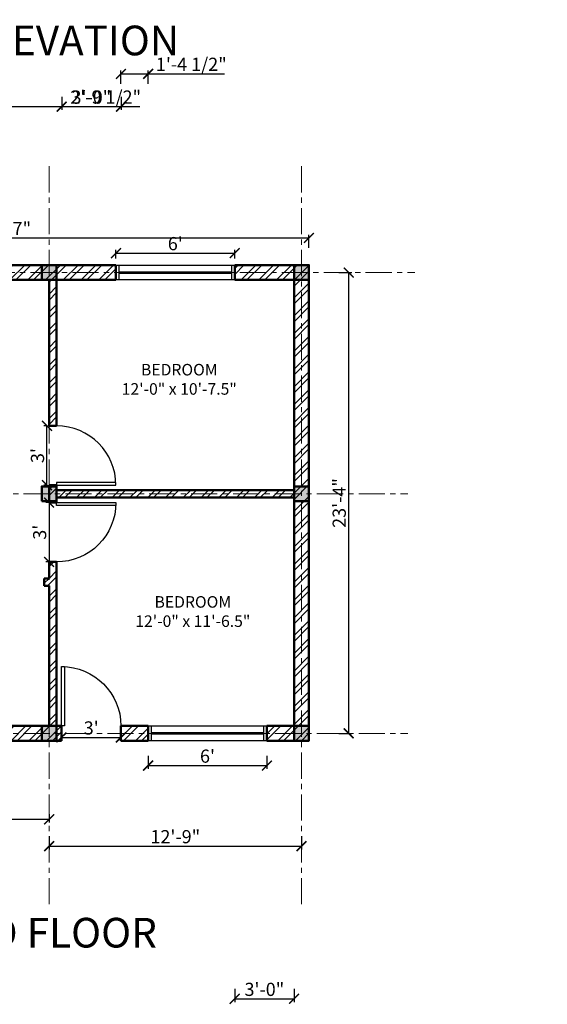
# Model space of a CAD drawing. Units: inches. Extents: x 378 to 1617, y 130 to 1256.
# Tile 2 of 5: x 708 to 1028, y 134 to 731. Entities that reach past the tile are written whole.
import ezdxf

# ---------------------------------------------------------------- set-up
doc = ezdxf.new("R2010")
doc.units = ezdxf.units.IN
doc.linetypes.add('CENTER', pattern=[50.8, 31.75, -6.35, 6.35, -6.35])
for name, color, linetype, lineweight in [('A-ANNO-TEXT', 7, 'Continuous', 25), ('A-AREA-IDEN', 3, 'Continuous', 18), ('Column Hatch', 1, 'Continuous', 13), ('Columns', 241, 'Continuous', 50), ('Dimensions', 153, 'Continuous', 18), ('Doors', 2, 'Continuous', 25), ('Grid lines', 7, 'CENTER', 18), ('Wall Hatch', 11, 'Continuous', 13), ('Walls', 220, 'Continuous', 50), ('Windows', 140, 'Continuous', 25)]:
    doc.layers.add(name, color=color, linetype=linetype, lineweight=lineweight)
doc.styles.get("Standard").update_dxf_attribs({"font": 'arial.ttf'})
doc.dimstyles.new('ISO-25', dxfattribs={"dimtxt": 8, "dimasz": 6, "dimexe": 2, "dimexo": 4, "dimtad": 1, "dimdec": 0, "dimlunit": 3, "dimtxsty": 'Standard', "dimblk": 'ARCHTICK', "dimcen": 2.5, "dimadec": 0, "dimazin": 0, "dimtfac": 1, "dimtdec": 0, "dimtmove": 0, "dimatfit": 3, "dimfxl": 6, "dimfxlon": 1, "dimarcsym": 0})

# ---------------------------------------------------------------- blocks, each defined once
blk = doc.blocks.new('*U5')
for p, q in [((0, 0), (0, -4)), ((-36, 0), (-36, -4))]:
    blk.add_line(p, q)
blk.add_lwpolyline([(0, 0), (0, 36), (-1.75, 36), (-1.75, 0)], close=True)
blk.add_arc((0, 0), 36, 90, 180)
blk = doc.blocks.new('*U6')
for p, q in [((0, 0), (0, -4)), ((-36, 0), (-36, -4))]:
    blk.add_line(p, q)
blk.add_lwpolyline([(0, 0), (0, 36), (-1.75, 36), (-1.75, 0)], close=True)
blk.add_arc((0, 0), 36, 90, 180)
blk = doc.blocks.new('_ArchTick')
at = {"color": 0, "linetype": 'ByBlock', "const_width": 0.15}
blk.add_lwpolyline([(-0.5, -0.5), (0.5, 0.5)], dxfattribs=at)
blk = doc.blocks.new('*D9')
at = {"layer": 'Defpoints', "color": 0, "transparency": 16777216}
for p in [(614.03, 252.95), (726.03, 252.95), (726.03, 245.84)]:
    blk.add_point(p, dxfattribs=at)
at = {"layer": 'Dimensions', "color": 0, "lineweight": -2, "transparency": 16777216}
for p, q in [((614.03, 248.95), (614.03, 243.84)), ((614.03, 245.84), (726.03, 245.84)), ((726.03, 248.95), (726.03, 243.84))]:
    blk.add_line(p, q, dxfattribs=at)
at = {"layer": 'Dimensions', "color": 0, "lineweight": -2, "transparency": 16777216, "xscale": 6, "yscale": 6, "zscale": 6, "rotation": 180}
blk.add_blockref('_ArchTick', (614.03, 245.84), dxfattribs=at)
at = {"layer": 'Dimensions', "color": 0, "lineweight": -2, "transparency": 16777216, "xscale": 6, "yscale": 6, "zscale": 6}
blk.add_blockref('_ArchTick', (726.03, 245.84), dxfattribs=at)
at = {"layer": 'Dimensions', "color": 0, "transparency": 16777216, "insert": (670.03, 250.55), "char_height": 8, "attachment_point": 5}
blk.add_mtext('9\'-4"', dxfattribs=at)
blk = doc.blocks.new('*D10')
at = {"layer": 'Defpoints', "color": 0, "transparency": 16777216}
for p in [(726.03, 293.45), (879.03, 293.45), (879.03, 229.55)]:
    blk.add_point(p, dxfattribs=at)
at = {"layer": 'Dimensions', "color": 0, "lineweight": -2, "transparency": 16777216}
for p, q in [((726.03, 235.55), (726.03, 227.55)), ((879.03, 235.55), (879.03, 227.55)), ((726.03, 229.55), (879.03, 229.55))]:
    blk.add_line(p, q, dxfattribs=at)
at = {"layer": 'Dimensions', "color": 0, "lineweight": -2, "transparency": 16777216, "xscale": 6, "yscale": 6, "zscale": 6, "rotation": 180}
blk.add_blockref('_ArchTick', (726.03, 229.55), dxfattribs=at)
at = {"layer": 'Dimensions', "color": 0, "lineweight": -2, "transparency": 16777216, "xscale": 6, "yscale": 6, "zscale": 6}
blk.add_blockref('_ArchTick', (879.03, 229.55), dxfattribs=at)
at = {"layer": 'Dimensions', "color": 0, "transparency": 16777216, "insert": (802.53, 234.26), "char_height": 8, "attachment_point": 5}
blk.add_mtext('12\'-9"', dxfattribs=at)
blk = doc.blocks.new('*D13')
at = {"layer": 'Defpoints', "color": 0, "transparency": 16777216}
for p in [(883.53, 577.45), (907.65, 577.45), (883.53, 297.95)]:
    blk.add_point(p, dxfattribs=at)
at = {"layer": 'Dimensions', "color": 0, "lineweight": -2, "transparency": 16777216}
for p, q in [((901.65, 577.45), (909.65, 577.45)), ((907.65, 297.95), (907.65, 577.45)), ((901.65, 297.95), (909.65, 297.95))]:
    blk.add_line(p, q, dxfattribs=at)
at = {"layer": 'Dimensions', "color": 0, "lineweight": -2, "transparency": 16777216, "xscale": 6, "yscale": 6, "zscale": 6}
for p, rotation in [((907.65, 577.45), 90), ((907.65, 297.95), 270)]:
    blk.add_blockref('_ArchTick', p, dxfattribs=dict(at, rotation=rotation))
at = {"layer": 'Dimensions', "color": 0, "transparency": 16777216, "insert": (902.94, 437.7), "char_height": 8, "attachment_point": 5, "rotation": 90}
blk.add_mtext('23\'-4"', dxfattribs=at)
blk = doc.blocks.new('*D14')
at = {"layer": 'Defpoints', "color": 0, "transparency": 16777216}
for p in [(883.53, 598.41), (516.53, 581.95), (883.53, 581.95)]:
    blk.add_point(p, dxfattribs=at)
at = {"layer": 'Dimensions', "color": 0, "lineweight": -2, "transparency": 16777216}
for p, q in [((516.53, 592.41), (516.53, 600.41)), ((516.53, 598.41), (883.53, 598.41)), ((883.53, 592.41), (883.53, 600.41))]:
    blk.add_line(p, q, dxfattribs=at)
at = {"layer": 'Dimensions', "color": 0, "lineweight": -2, "transparency": 16777216, "xscale": 6, "yscale": 6, "zscale": 6, "rotation": 180}
blk.add_blockref('_ArchTick', (516.53, 598.41), dxfattribs=at)
at = {"layer": 'Dimensions', "color": 0, "lineweight": -2, "transparency": 16777216, "xscale": 6, "yscale": 6, "zscale": 6}
blk.add_blockref('_ArchTick', (883.53, 598.41), dxfattribs=at)
at = {"layer": 'Dimensions', "color": 0, "transparency": 16777216, "insert": (700.03, 603.12), "char_height": 8, "attachment_point": 5}
blk.add_mtext('30\'-7"', dxfattribs=at)
blk = doc.blocks.new('*D26')
at = {"layer": 'Defpoints', "color": 0, "transparency": 16777216}
for p in [(838.53, 589.23), (766.53, 581.95), (838.53, 581.95)]:
    blk.add_point(p, dxfattribs=at)
at = {"layer": 'Dimensions', "color": 0, "lineweight": -2, "transparency": 16777216}
for p, q in [((766.53, 585.95), (766.53, 591.23)), ((838.53, 585.95), (838.53, 591.23)), ((766.53, 589.23), (838.53, 589.23))]:
    blk.add_line(p, q, dxfattribs=at)
at = {"layer": 'Dimensions', "color": 0, "lineweight": -2, "transparency": 16777216, "xscale": 6, "yscale": 6, "zscale": 6, "rotation": 180}
blk.add_blockref('_ArchTick', (766.53, 589.23), dxfattribs=at)
at = {"layer": 'Dimensions', "color": 0, "lineweight": -2, "transparency": 16777216, "xscale": 6, "yscale": 6, "zscale": 6}
blk.add_blockref('_ArchTick', (838.53, 589.23), dxfattribs=at)
at = {"layer": 'Dimensions', "color": 0, "transparency": 16777216, "insert": (802.53, 593.94), "char_height": 8, "attachment_point": 5}
blk.add_mtext("6'", dxfattribs=at)
blk = doc.blocks.new('*D27')
at = {"layer": 'Defpoints', "color": 0, "transparency": 16777216}
for p in [(786.03, 293.45), (858.03, 293.45), (858.03, 278.41)]:
    blk.add_point(p, dxfattribs=at)
at = {"layer": 'Dimensions', "color": 0, "lineweight": -2, "transparency": 16777216}
for p, q in [((786.03, 284.41), (786.03, 276.41)), ((858.03, 284.41), (858.03, 276.41)), ((786.03, 278.41), (858.03, 278.41))]:
    blk.add_line(p, q, dxfattribs=at)
at = {"layer": 'Dimensions', "color": 0, "lineweight": -2, "transparency": 16777216, "xscale": 6, "yscale": 6, "zscale": 6, "rotation": 180}
blk.add_blockref('_ArchTick', (786.03, 278.41), dxfattribs=at)
at = {"layer": 'Dimensions', "color": 0, "lineweight": -2, "transparency": 16777216, "xscale": 6, "yscale": 6, "zscale": 6}
blk.add_blockref('_ArchTick', (858.03, 278.41), dxfattribs=at)
at = {"layer": 'Dimensions', "color": 0, "transparency": 16777216, "insert": (822.03, 283.12), "char_height": 8, "attachment_point": 5}
blk.add_mtext("6'", dxfattribs=at)
blk = doc.blocks.new('*D29')
at = {"layer": 'Defpoints', "color": 0, "transparency": 16777216}
for p in [(733.53, 297.95), (769.53, 297.95), (769.53, 295.49)]:
    blk.add_point(p, dxfattribs=at)
at = {"layer": 'Dimensions', "color": 0, "lineweight": -2, "transparency": 16777216}
for p, q in [((733.53, 295.49), (733.53, 293.49)), ((733.53, 295.49), (769.53, 295.49)), ((769.53, 295.49), (769.53, 293.49))]:
    blk.add_line(p, q, dxfattribs=at)
at = {"layer": 'Dimensions', "color": 0, "lineweight": -2, "transparency": 16777216, "xscale": 6, "yscale": 6, "zscale": 6, "rotation": 180}
blk.add_blockref('_ArchTick', (733.53, 295.49), dxfattribs=at)
at = {"layer": 'Dimensions', "color": 0, "lineweight": -2, "transparency": 16777216, "xscale": 6, "yscale": 6, "zscale": 6}
blk.add_blockref('_ArchTick', (769.53, 295.49), dxfattribs=at)
at = {"layer": 'Dimensions', "color": 0, "transparency": 16777216, "insert": (751.53, 300.21), "char_height": 8, "attachment_point": 5}
blk.add_mtext("3'", dxfattribs=at)
blk = doc.blocks.new('*D30')
at = {"layer": 'Defpoints', "color": 0, "transparency": 16777216}
for p in [(728.53, 437.95), (726.03, 401.95), (728.53, 401.95)]:
    blk.add_point(p, dxfattribs=at)
at = {"layer": 'Dimensions', "color": 0, "lineweight": -2, "transparency": 16777216}
for p, q in [((726.03, 437.95), (724.03, 437.95)), ((726.03, 437.95), (726.03, 401.95)), ((726.03, 401.95), (724.03, 401.95))]:
    blk.add_line(p, q, dxfattribs=at)
at = {"layer": 'Dimensions', "color": 0, "lineweight": -2, "transparency": 16777216, "xscale": 6, "yscale": 6, "zscale": 6}
for p, rotation in [((726.03, 437.95), 90), ((726.03, 401.95), 270)]:
    blk.add_blockref('_ArchTick', p, dxfattribs=dict(at, rotation=rotation))
at = {"layer": 'Dimensions', "color": 0, "transparency": 16777216, "insert": (721.32, 419.95), "char_height": 8, "attachment_point": 5, "rotation": 90}
blk.add_mtext("3'", dxfattribs=at)
blk = doc.blocks.new('*D34')
at = {"layer": 'Defpoints', "color": 0, "transparency": 16777216}
for p in [(724.72, 484.45), (728.28, 484.45), (728.28, 448.45)]:
    blk.add_point(p, dxfattribs=at)
at = {"layer": 'Dimensions', "color": 0, "lineweight": -2, "transparency": 16777216}
for p, q in [((724.72, 484.45), (722.72, 484.45)), ((724.72, 448.45), (724.72, 484.45)), ((724.72, 448.45), (722.72, 448.45))]:
    blk.add_line(p, q, dxfattribs=at)
at = {"layer": 'Dimensions', "color": 0, "lineweight": -2, "transparency": 16777216, "xscale": 6, "yscale": 6, "zscale": 6}
for p, rotation in [((724.72, 484.45), 90), ((724.72, 448.45), 270)]:
    blk.add_blockref('_ArchTick', p, dxfattribs=dict(at, rotation=rotation))
at = {"layer": 'Dimensions', "color": 0, "transparency": 16777216, "insert": (720.01, 466.45), "char_height": 8, "attachment_point": 5, "rotation": 90}
blk.add_mtext("3'", dxfattribs=at)
blk = doc.blocks.new('*D58')
at = {"layer": 'Defpoints', "color": 0, "transparency": 16777216}
for p in [(838.53, 572.95), (874.53, 572.95), (874.53, 136.95)]:
    blk.add_point(p, dxfattribs=at)
at = {"layer": 'Dimensions', "color": 0, "lineweight": -2, "transparency": 16777216}
for p, q in [((838.53, 142.95), (838.53, 134.95)), ((874.53, 142.95), (874.53, 134.95)), ((838.53, 136.95), (874.53, 136.95))]:
    blk.add_line(p, q, dxfattribs=at)
at = {"layer": 'Dimensions', "color": 0, "lineweight": -2, "transparency": 16777216, "xscale": 6, "yscale": 6, "zscale": 6, "rotation": 180}
blk.add_blockref('_ArchTick', (838.53, 136.95), dxfattribs=at)
at = {"layer": 'Dimensions', "color": 0, "lineweight": -2, "transparency": 16777216, "xscale": 6, "yscale": 6, "zscale": 6}
blk.add_blockref('_ArchTick', (874.53, 136.95), dxfattribs=at)
at = {"layer": 'Dimensions', "color": 0, "transparency": 16777216, "insert": (856.53, 141.66), "char_height": 8, "attachment_point": 5}
blk.add_mtext('3\'-0"', dxfattribs=at)
blk = doc.blocks.new('*D60')
at = {"layer": 'Defpoints', "color": 0, "transparency": 16777216}
for p in [(786.03, 697.95), (769.53, 302.45), (786.03, 302.45)]:
    blk.add_point(p, dxfattribs=at)
at = {"layer": 'Dimensions', "color": 0, "lineweight": -2, "transparency": 16777216}
for p, q in [((769.53, 691.95), (769.53, 699.95)), ((786.03, 691.95), (786.03, 699.95)), ((769.53, 697.95), (786.03, 697.95)), ((786.03, 697.95), (832.43, 697.95))]:
    blk.add_line(p, q, dxfattribs=at)
at = {"layer": 'Dimensions', "color": 0, "lineweight": -2, "transparency": 16777216, "xscale": 6, "yscale": 6, "zscale": 6, "rotation": 180}
blk.add_blockref('_ArchTick', (769.53, 697.95), dxfattribs=at)
at = {"layer": 'Dimensions', "color": 0, "lineweight": -2, "transparency": 16777216, "xscale": 6, "yscale": 6, "zscale": 6}
blk.add_blockref('_ArchTick', (786.03, 697.95), dxfattribs=at)
at = {"layer": 'Dimensions', "color": 0, "transparency": 16777216, "insert": (812.23, 702.71), "char_height": 8, "attachment_point": 5}
blk.add_mtext('1\'-4 1/2"', dxfattribs=at)
blk = doc.blocks.new('*D77')
at = {"layer": 'Defpoints', "color": 0, "transparency": 16777216}
for p in [(733.65, 812.09), (769.65, 812.09), (769.65, 678.08)]:
    blk.add_point(p, dxfattribs=at)
at = {"layer": 'Dimensions', "color": 0, "lineweight": -2, "transparency": 16777216}
for p, q in [((733.65, 684.08), (733.65, 676.08)), ((769.65, 684.08), (769.65, 676.08)), ((733.65, 678.08), (769.65, 678.08))]:
    blk.add_line(p, q, dxfattribs=at)
at = {"layer": 'Dimensions', "color": 0, "lineweight": -2, "transparency": 16777216, "xscale": 6, "yscale": 6, "zscale": 6, "rotation": 180}
blk.add_blockref('_ArchTick', (733.65, 678.08), dxfattribs=at)
at = {"layer": 'Dimensions', "color": 0, "lineweight": -2, "transparency": 16777216, "xscale": 6, "yscale": 6, "zscale": 6}
blk.add_blockref('_ArchTick', (769.65, 678.08), dxfattribs=at)
at = {"layer": 'Dimensions', "color": 0, "transparency": 16777216, "insert": (751.65, 682.79), "char_height": 8, "attachment_point": 5}
blk.add_mtext('3\'-0"', dxfattribs=at)
blk = doc.blocks.new('*D82')
at = {"layer": 'Defpoints', "color": 0, "transparency": 16777216}
for p in [(700.03, 851.08), (733.65, 812.09), (733.65, 678.08)]:
    blk.add_point(p, dxfattribs=at)
at = {"layer": 'Dimensions', "color": 0, "lineweight": -2, "transparency": 16777216}
for p, q in [((700.03, 684.08), (700.03, 676.08)), ((733.65, 684.08), (733.65, 676.08)), ((700.03, 678.08), (733.65, 678.08)), ((733.65, 678.08), (780.95, 678.08))]:
    blk.add_line(p, q, dxfattribs=at)
at = {"layer": 'Dimensions', "color": 0, "lineweight": -2, "transparency": 16777216, "xscale": 6, "yscale": 6, "zscale": 6, "rotation": 180}
blk.add_blockref('_ArchTick', (700.03, 678.08), dxfattribs=at)
at = {"layer": 'Dimensions', "color": 0, "lineweight": -2, "transparency": 16777216, "xscale": 6, "yscale": 6, "zscale": 6}
blk.add_blockref('_ArchTick', (733.65, 678.08), dxfattribs=at)
at = {"layer": 'Dimensions', "color": 0, "transparency": 16777216, "insert": (760.3, 682.84), "char_height": 8, "attachment_point": 5}
blk.add_mtext('2\'-9 1/2"', dxfattribs=at)

msp = doc.modelspace()

# ---------------------------------------------------------------- hatches: boundary and pattern name
at = {"layer": 'Column Hatch'}
h = msp.add_hatch(color=256, dxfattribs=at)
h.dxf.hatch_style = 1
h.paths.add_polyline_path([(525.53, 581.95), (516.53, 581.95), (516.53, 572.95), (525.53, 572.95)])
h.paths.add_polyline_path([(618.53, 581.95), (609.53, 581.95), (609.53, 572.95), (618.53, 572.95)])
h.paths.add_polyline_path([(730.53, 581.95), (721.53, 581.95), (721.53, 572.95), (730.53, 572.95)])
h.paths.add_polyline_path([(883.53, 581.95), (874.53, 581.95), (874.53, 572.95), (883.53, 572.95)])
h.paths.add_polyline_path([(883.53, 447.7), (874.53, 447.7), (874.53, 438.7), (883.53, 438.7)])
h.paths.add_polyline_path([(730.53, 447.7), (721.53, 447.7), (721.53, 438.7), (730.53, 438.7)])
h.paths.add_polyline_path([(618.53, 447.7), (609.53, 447.7), (609.53, 438.7), (618.53, 438.7)])
h.paths.add_polyline_path([(525.53, 447.7), (516.53, 447.7), (516.53, 438.7), (525.53, 438.7)])
h.paths.add_polyline_path([(525.53, 302.45), (516.53, 302.45), (516.53, 293.45), (525.53, 293.45)])
h.paths.add_polyline_path([(618.53, 302.45), (609.53, 302.45), (609.53, 293.45), (618.53, 293.45)])
h.paths.add_polyline_path([(730.53, 302.45), (721.53, 302.45), (721.53, 293.45), (730.53, 293.45)])
h.paths.add_polyline_path([(883.53, 302.45), (874.53, 302.45), (874.53, 293.45), (883.53, 293.45)])
h.paths.add_polyline_path([(1125.53, 302.45), (1116.53, 302.45), (1116.53, 293.45), (1125.53, 293.45)])
h.paths.add_polyline_path([(1218.53, 302.45), (1209.53, 302.45), (1209.53, 293.45), (1218.53, 293.45)])
h.paths.add_polyline_path([(1330.53, 302.45), (1321.53, 302.45), (1321.53, 293.45), (1330.53, 293.45)])
h.paths.add_polyline_path([(1483.53, 302.45), (1474.53, 302.45), (1474.53, 293.45), (1483.53, 293.45)])
h.paths.add_polyline_path([(1483.53, 447.7), (1474.53, 447.7), (1474.53, 438.7), (1483.53, 438.7)])
h.paths.add_polyline_path([(1330.53, 447.7), (1321.53, 447.7), (1321.53, 438.7), (1330.53, 438.7)])
h.paths.add_polyline_path([(1218.53, 447.7), (1209.53, 447.7), (1209.53, 438.7), (1218.53, 438.7)])
h.paths.add_polyline_path([(1125.53, 447.7), (1116.53, 447.7), (1116.53, 438.7), (1125.53, 438.7)])
h.paths.add_polyline_path([(1125.53, 581.95), (1116.53, 581.95), (1116.53, 572.95), (1125.53, 572.95)])
h.paths.add_polyline_path([(1218.53, 581.95), (1209.53, 581.95), (1209.53, 572.95), (1218.53, 572.95)])
h.paths.add_polyline_path([(1330.53, 581.95), (1321.53, 581.95), (1321.53, 572.95), (1330.53, 572.95)])
h.paths.add_polyline_path([(1483.53, 581.95), (1474.53, 581.95), (1474.53, 572.95), (1483.53, 572.95)])
at = {"layer": 'Wall Hatch'}
h = msp.add_hatch(dxfattribs=at)
h.set_pattern_fill('ANSI32', color=256, scale=0.8)
h.paths.add_polyline_path([(525.53, 493.45), (609.53, 493.45), (609.53, 490.45), (614.03, 490.45), (614.03, 500.95), (609.53, 500.95), (609.53, 497.95), (525.53, 497.95), (525.53, 572.95), (527.53, 572.95), (527.53, 581.95), (516.53, 581.95), (516.53, 252.95), (614.03, 252.95), (614.03, 293.45), (609.53, 293.45), (609.53, 257.45), (525.53, 257.45), (525.53, 297.95), (609.53, 297.95), (609.53, 302.45), (525.53, 302.45), (525.53, 440.95), (609.53, 440.95), (609.53, 435.7), (614.03, 435.7), (614.03, 466.45), (609.53, 466.45), (609.53, 445.45), (525.53, 445.45)])
h.paths.add_polyline_path([(640.03, 302.45), (614.03, 302.45), (614.03, 387.45), (693.03, 387.45), (693.03, 391.95), (614.03, 391.95), (614.03, 393.7), (609.53, 393.7), (609.53, 293.45), (640.03, 293.45)])
h.paths.add_polyline_path([(733.53, 302.45), (730.53, 302.45), (730.53, 401.95), (726.03, 401.95), (726.03, 391.95), (723.03, 391.95), (723.03, 387.45), (726.03, 387.45), (726.03, 302.45), (700.03, 302.45), (700.03, 293.45), (733.53, 293.45)])
h.paths.add_polyline_path([(883.53, 581.95), (838.53, 581.95), (838.53, 572.95), (874.53, 572.95), (874.53, 445.45), (730.53, 445.45), (730.53, 448.45), (726.03, 448.45), (726.03, 437.95), (730.53, 437.95), (730.53, 440.95), (874.53, 440.95), (874.53, 302.45), (858.03, 302.45), (858.03, 293.45), (883.53, 293.45)])
h.paths.add_polyline_path([(730.53, 572.95), (766.53, 572.95), (766.53, 581.95), (694.03, 581.95), (694.03, 572.95), (726.03, 572.95), (726.03, 484.45), (730.53, 484.45)])
h.paths.add_polyline_path([(646.03, 581.95), (551.53, 581.95), (551.53, 572.95), (609.53, 572.95), (609.53, 530.95), (614.03, 530.95), (614.03, 572.95), (646.03, 572.95)])
h.paths.add_polyline_path([(786.03, 302.45), (769.53, 302.45), (769.53, 293.45), (786.03, 293.45)], flags=17)

# ---------------------------------------------------------------- linework, layer by layer
at = {"layer": 'Columns'}
for points in [[(721.53, 572.95), (730.53, 572.95), (730.53, 581.95), (721.53, 581.95)], [(874.53, 572.95), (883.53, 572.95), (883.53, 581.95), (874.53, 581.95)], [(721.53, 438.7), (730.53, 438.7), (730.53, 447.7), (721.53, 447.7)], [(874.53, 438.7), (883.53, 438.7), (883.53, 447.7), (874.53, 447.7)], [(721.53, 293.45), (730.53, 293.45), (730.53, 302.45), (721.53, 302.45)], [(874.53, 293.45), (883.53, 293.45), (883.53, 302.45), (874.53, 302.45)]]:
    msp.add_lwpolyline(points, close=True, dxfattribs=at)
at = {"layer": 'Grid lines', "ltscale": 0.5}
for p, q in [((726.03, 641.95), (726.03, 192.95)), ((879.03, 641.95), (879.03, 192.95)), ((460.71, 577.45), (947.71, 577.45)), ((456.53, 443.2), (943.53, 443.2)), ((456.53, 297.95), (943.53, 297.95))]:
    msp.add_line(p, q, dxfattribs=at)
at = {"layer": 'Walls'}
for p, q in [((694.03, 581.95), (766.53, 581.95)), ((766.53, 572.95), (766.53, 581.95)), ((838.53, 572.95), (838.53, 581.95)), ((838.53, 581.95), (883.53, 581.95)), ((883.53, 581.95), (883.53, 293.45)), ((694.03, 572.95), (726.03, 572.95)), ((726.03, 572.95), (726.03, 484.45)), ((730.53, 572.95), (730.53, 484.45)), ((730.53, 572.95), (766.53, 572.95)), ((838.53, 572.95), (874.53, 572.95)), ((874.53, 572.95), (874.53, 445.45)), ((730.53, 484.45), (726.03, 484.45)), ((730.53, 448.45), (726.03, 448.45)), ((726.03, 448.45), (726.03, 437.95)), ((730.53, 448.45), (730.53, 445.45)), ((730.53, 445.45), (874.53, 445.45)), ((730.53, 437.95), (726.03, 437.95)), ((730.53, 440.95), (730.53, 437.95)), ((730.53, 440.95), (874.53, 440.95)), ((874.53, 440.95), (874.53, 302.45)), ((730.53, 401.95), (726.03, 401.95)), ((726.03, 401.95), (726.03, 391.95)), ((730.53, 401.95), (730.53, 302.45)), ((723.03, 391.95), (723.03, 387.45)), ((723.03, 391.95), (726.03, 391.95)), ((723.03, 387.45), (726.03, 387.45)), ((726.03, 387.45), (726.03, 302.45)), ((700.03, 302.45), (726.03, 302.45)), ((730.53, 302.45), (733.53, 302.45)), ((733.53, 302.45), (733.53, 293.45)), ((769.53, 302.45), (769.53, 293.45)), ((769.53, 302.45), (786.03, 302.45)), ((786.03, 302.45), (786.03, 293.45)), ((858.03, 302.45), (858.03, 293.45)), ((858.03, 302.45), (874.53, 302.45)), ((700.03, 293.45), (733.53, 293.45)), ((769.53, 293.45), (786.03, 293.45)), ((858.03, 293.45), (883.53, 293.45))]:
    msp.add_line(p, q, dxfattribs=at)
at = {"layer": 'Windows'}
for p, q in [((766.53, 572.95), (766.53, 581.95)), ((766.53, 581.95), (838.53, 581.95)), ((768.53, 572.95), (768.53, 581.95)), ((836.53, 581.95), (836.53, 572.95)), ((838.53, 581.95), (838.53, 572.95)), ((768.53, 577.95), (836.53, 577.95)), ((836.53, 576.95), (768.53, 576.95)), ((838.53, 572.95), (766.53, 572.95)), ((786.03, 293.45), (786.03, 302.45)), ((786.03, 302.45), (858.03, 302.45)), ((788.03, 293.45), (788.03, 302.45)), ((856.03, 302.45), (856.03, 293.45)), ((858.03, 302.45), (858.03, 293.45)), ((858.03, 293.45), (786.03, 293.45)), ((788.03, 298.45), (856.03, 298.45)), ((856.03, 297.45), (788.03, 297.45))]:
    msp.add_line(p, q, dxfattribs=at)

# ---------------------------------------------------------------- block references
at = {"layer": 'Doors', "rotation": 270}
msp.add_blockref('*U5', (730.53, 448.45), dxfattribs=at)
at = {"layer": 'Doors', "xscale": -1}
for name, p, rotation in [('*U5', (730.53, 437.95), 269.9999999999999), ('*U6', (733.53, 302.45), 359.9999999999999)]:
    msp.add_blockref(name, p, dxfattribs=dict(at, rotation=rotation))

# ---------------------------------------------------------------- texts
at = {"layer": 'A-ANNO-TEXT', "char_height": 18, "attachment_point": 1}
for s, insert in [('\\pxqc;{\\fTimes New Roman|b0|i0|c0|p18;FRONT ELEVATION}', (524.62, 727.2)), ('\\pxqc;{\\fTimes New Roman|b0|i0|c0|p18;GROUND FLOOR}', (524.62, 186.07))]:
    msp.add_mtext_dynamic_manual_height_columns(s, width=345.962, gutter_width=12.5, heights=[0], dxfattribs=dict(at, insert=insert))
at = {"layer": 'A-AREA-IDEN', "char_height": 7, "attachment_point": 1}
for s, width, insert in [('\\pxqc;{\\fTimes New Roman|b0|i0|c0|p18;BEDROOM\\P12\'-0" x 10\'-7.5"}', 73.2905, (768.28, 522.03)), ('\\pxqc;{\\fTimes New Roman|b0|i0|c0|p18;BEDROOM\\P12\'-0" x 11\'-6.5"}', 70.4926, (777.89, 381.18))]:
    msp.add_mtext_dynamic_manual_height_columns(s, width=width, gutter_width=12.5, heights=[0], dxfattribs=dict(at, insert=insert))

# ---------------------------------------------------------------- dimensions: what is measured, and where the dimension line sits
at = {"layer": 'Dimensions'}
for base, p1, p2, override, picture, middle in [((733.65, 678.08), (700.03, 851.08), (733.65, 812.09), {"dimdec": 1, "dimlfac": 1, "dimrnd": 0, "dimzin": 1, "dimdsep": 46, "dimlunit": 4, "dimfrac": 2}, '*D82', (760.3, 682.84)), ((769.65, 678.08), (733.65, 812.09), (769.65, 812.09), {"dimdec": 1, "dimlfac": 1, "dimrnd": 0, "dimzin": 1, "dimdsep": 46, "dimlunit": 4, "dimfrac": 2}, '*D77', (751.65, 682.79)), ((786.03, 697.95), (769.53, 302.45), (786.03, 302.45), {"dimdec": 1, "dimlfac": 1, "dimrnd": 0, "dimzin": 1, "dimdsep": 46, "dimlunit": 4, "dimfrac": 2}, '*D60', (812.23, 702.71)), ((883.53, 598.41), (516.53, 581.95), (883.53, 581.95), {"dimclrd": 0, "dimclre": 0, "dimclrt": 0}, '*D14', (700.03, 603.12)), ((838.53, 589.23), (766.53, 581.95), (838.53, 581.95), {"dimclrd": 0, "dimclre": 0, "dimclrt": 0}, '*D26', (802.53, 593.94)), ((874.53, 136.95), (838.53, 572.95), (874.53, 572.95), {"dimdec": 1, "dimlfac": 1, "dimrnd": 0, "dimzin": 1, "dimdsep": 46, "dimlunit": 4, "dimfrac": 2}, '*D58', (856.53, 141.66)), ((769.53, 295.49), (733.53, 297.95), (769.53, 297.95), {"dimclrd": 0, "dimclre": 0, "dimclrt": 0}, '*D29', (751.53, 300.21)), ((879.03, 229.55), (726.03, 293.45), (879.03, 293.45), {"dimclrd": 0, "dimclre": 0, "dimclrt": 0}, '*D10', (802.53, 234.26)), ((858.03, 278.41), (786.03, 293.45), (858.03, 293.45), {"dimclrd": 0, "dimclre": 0, "dimclrt": 0}, '*D27', (822.03, 283.12)), ((726.03, 245.84), (614.03, 252.95), (726.03, 252.95), {"dimclrd": 0, "dimclre": 0, "dimclrt": 0}, '*D9', (670.03, 250.55))]:
    dim = msp.add_linear_dim(base=base, p1=p1, p2=p2, dimstyle='ISO-25', override=override, dxfattribs=at)
    dim.commit()
    dim.dimension.update_dxf_attribs({"geometry": picture, "text_midpoint": middle})
for base, p1, p2, picture, middle in [((907.64846102, 577.45088562), (883.5278532, 297.95088562), (883.5278532, 577.45088562), '*D13', (902.9361486, 437.70088562)), ((724.72, 484.45), (728.28, 448.45), (728.28, 484.45), '*D34', (720.01, 466.45)), ((726.03, 401.95), (728.53, 437.95), (728.53, 401.95), '*D30', (721.32, 419.95))]:
    dim = msp.add_linear_dim(base=base, p1=p1, p2=p2, angle=90, dimstyle='ISO-25', override={"dimclrd": 0, "dimclre": 0, "dimclrt": 0}, dxfattribs=at)
    dim.commit()
    dim.dimension.update_dxf_attribs({"geometry": picture, "text_midpoint": middle})

doc.saveas('drawing.dxf')
